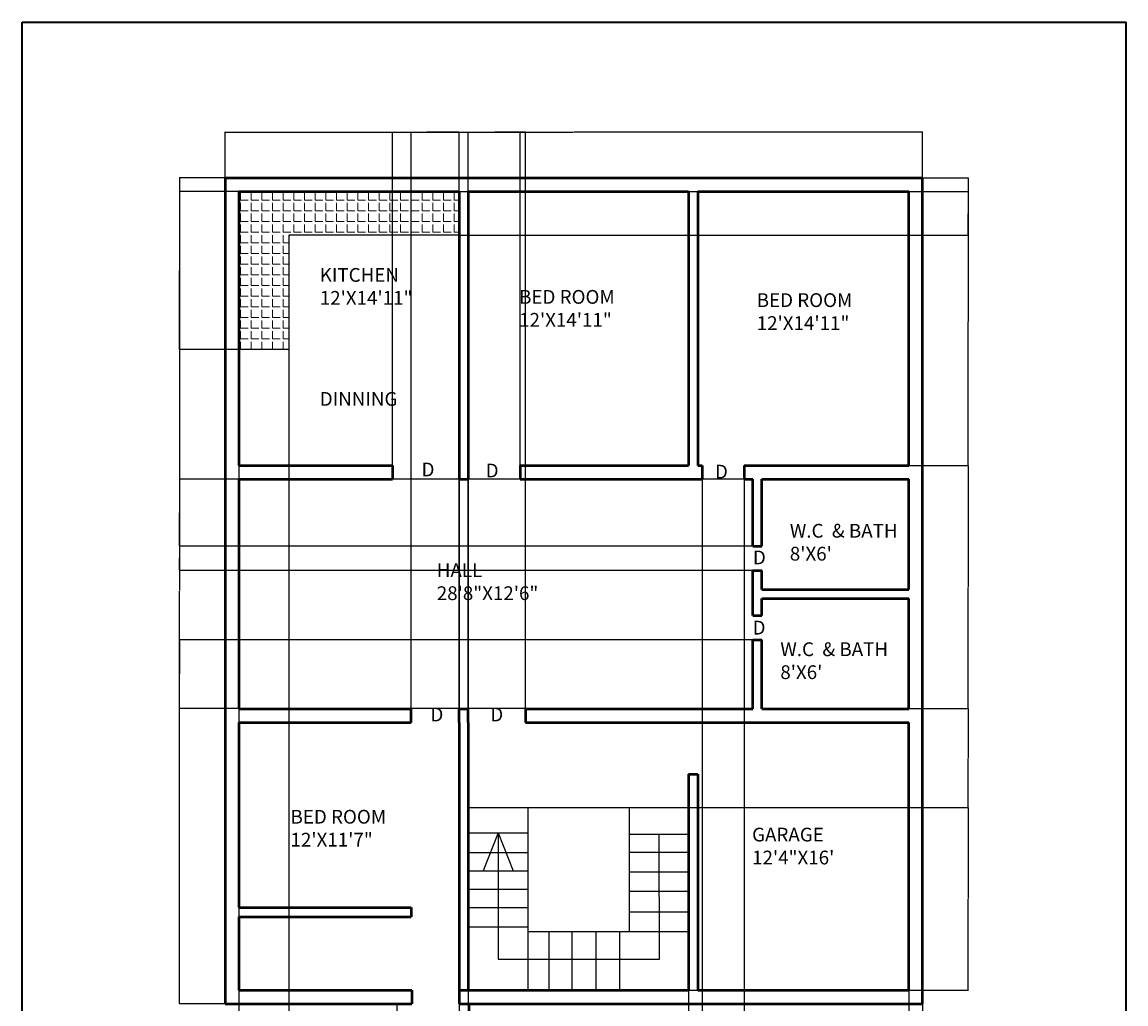
# Model space of a CAD drawing. Units: feet. Extents: x 3406 to 4127, y 2162 to 3204.
# Tile 3 of 3: x 3406 to 4127, y 2562 to 3204. Entities that reach past the tile are written whole.
import ezdxf

# ---------------------------------------------------------------- set-up
doc = ezdxf.new("R2010")
doc.units = ezdxf.units.FT
for name, color, linetype, lineweight in [('A-ANNO-DIMS', 2, 'Continuous', 18), ('A-ANNO-TEXT', 7, 'Continuous', 18), ('A-ANNO-TTLB', 7, 'Continuous', 35), ('A-AREA-IDEN', 7, 'Continuous', 18), ('A-FLOR-FIXT', 8, 'Continuous', 25), ('A-FLOR-FIXT-PATT', 9, 'Continuous', 13), ('A-FLOR-STRS', 7, 'Continuous', 25), ('A-WALL', 7, 'Continuous', 50)]:
    doc.layers.add(name, color=color, linetype=linetype, lineweight=lineweight)
doc.styles.get("Standard").update_dxf_attribs({"font": 'arial.ttf'})
doc.dimstyles.get("Standard").update_dxf_attribs({"dimtxt": 0.18, "dimasz": 0.18, "dimexe": 0.18, "dimexo": 0.0625, "dimgap": 0.09, "dimtad": 0, "dimtih": 1, "dimtoh": 1, "dimdec": 4, "dimzin": 0, "dimdsep": 46, "dimtxsty": 'Standard', "dimcen": 0.09, "dimadec": 0, "dimazin": 0, "dimtfac": 1, "dimtdec": 4, "dimtofl": 0, "dimtmove": 0, "dimatfit": 3, "dimfxl": 1, "dimtolj": 1, "dimtzin": 0, "dimarcsym": 0})

# ---------------------------------------------------------------- blocks, each defined once
blk = doc.blocks.new('*D4')
at = {"layer": 'A-ANNO-DIMS', "color": 0, "lineweight": -2, "transparency": 16777216}
for p, q in [((3538.39, 3101.97), (3538.39, 3131.89)), ((3994.39, 3101.97), (3994.39, 3131.89)), ((3538.57, 3131.71), (3766.1, 3131.71)), ((3994.21, 3131.71), (3766.68, 3131.71))]:
    blk.add_line(p, q, dxfattribs=at)
at = {"layer": 'A-ANNO-DIMS', "color": 0, "transparency": 16777216}
for points in [[(3538.57, 3131.74), (3538.57, 3131.68), (3538.39, 3131.71)], [(3994.21, 3131.74), (3994.21, 3131.68), (3994.39, 3131.71)]]:
    blk.add_solid(points, dxfattribs=at)
at = {"layer": 'Defpoints', "color": 0, "transparency": 16777216}
for p in [(3994.39, 3131.71), (3538.39, 3101.91), (3994.39, 3101.91)]:
    blk.add_point(p, dxfattribs=at)
at = {"layer": 'A-ANNO-DIMS', "color": 0, "transparency": 16777216, "insert": (3766.39, 3131.71), "char_height": 0.18, "attachment_point": 5}
blk.add_mtext('\\A1;456', dxfattribs=at)
blk = doc.blocks.new('*D5')
at = {"layer": 'A-ANNO-DIMS', "color": 0, "lineweight": -2, "transparency": 16777216}
for p, q in [((3538.33, 3101.91), (3508.41, 3101.91)), ((3508.59, 3101.73), (3508.59, 2832.09)), ((3508.59, 2562.09), (3508.59, 2831.72)), ((3538.33, 2561.91), (3508.41, 2561.91))]:
    blk.add_line(p, q, dxfattribs=at)
at = {"layer": 'A-ANNO-DIMS', "color": 0, "transparency": 16777216}
for points in [[(3508.56, 3101.73), (3508.62, 3101.73), (3508.59, 3101.91)], [(3508.56, 2562.09), (3508.62, 2562.09), (3508.59, 2561.91)]]:
    blk.add_solid(points, dxfattribs=at)
at = {"layer": 'Defpoints', "color": 0, "transparency": 16777216}
for p in [(3538.39, 3101.91), (3508.59, 2561.91), (3538.39, 2561.91)]:
    blk.add_point(p, dxfattribs=at)
at = {"layer": 'A-ANNO-DIMS', "color": 0, "transparency": 16777216, "insert": (3508.59, 2831.91), "char_height": 0.18, "attachment_point": 5}
blk.add_mtext('\\A1;540', dxfattribs=at)
blk = doc.blocks.new('*D9')
at = {"layer": 'A-ANNO-DIMS', "color": 0, "lineweight": -2, "transparency": 16777216}
for p, q in [((3841.39, 2570.84), (3841.39, 2509.54)), ((3985.39, 2570.84), (3985.39, 2509.54)), ((3841.57, 2509.72), (3913.11, 2509.72)), ((3985.21, 2509.72), (3913.67, 2509.72))]:
    blk.add_line(p, q, dxfattribs=at)
at = {"layer": 'A-ANNO-DIMS', "color": 0, "transparency": 16777216}
for points in [[(3841.57, 2509.75), (3841.57, 2509.69), (3841.39, 2509.72)], [(3985.21, 2509.75), (3985.21, 2509.69), (3985.39, 2509.72)]]:
    blk.add_solid(points, dxfattribs=at)
at = {"layer": 'Defpoints', "color": 0, "transparency": 16777216}
for p in [(3841.39, 2570.91), (3985.39, 2570.91), (3985.39, 2509.72)]:
    blk.add_point(p, dxfattribs=at)
at = {"layer": 'A-ANNO-DIMS', "color": 0, "transparency": 16777216, "insert": (3913.39, 2509.72), "char_height": 0.18, "attachment_point": 5}
blk.add_mtext('\\A1;144', dxfattribs=at)
blk = doc.blocks.new('*D10')
at = {"layer": 'A-ANNO-DIMS', "color": 0, "lineweight": -2, "transparency": 16777216}
for p, q in [((3994.45, 3101.91), (4024.37, 3101.91)), ((4024.19, 3101.73), (4024.19, 3008.09)), ((4024.19, 2914.09), (4024.19, 3007.72)), ((3985.45, 2913.91), (4024.37, 2913.91))]:
    blk.add_line(p, q, dxfattribs=at)
at = {"layer": 'A-ANNO-DIMS', "color": 0, "transparency": 16777216}
for points in [[(4024.16, 3101.73), (4024.22, 3101.73), (4024.19, 3101.91)], [(4024.16, 2914.09), (4024.22, 2914.09), (4024.19, 2913.91)]]:
    blk.add_solid(points, dxfattribs=at)
at = {"layer": 'Defpoints', "color": 0, "transparency": 16777216}
for p in [(3994.39, 3101.91), (3985.39, 2913.91), (4024.19, 2913.91)]:
    blk.add_point(p, dxfattribs=at)
at = {"layer": 'A-ANNO-DIMS', "color": 0, "transparency": 16777216, "insert": (4024.19, 3007.91), "char_height": 0.18, "attachment_point": 5}
blk.add_mtext('\\A1;188', dxfattribs=at)
blk = doc.blocks.new('*D11')
at = {"layer": 'A-ANNO-DIMS', "color": 0, "lineweight": -2, "transparency": 16777216}
for p, q in [((3985.45, 2913.91), (4024.37, 2913.91)), ((4024.19, 2913.73), (4024.19, 2834.59)), ((4024.19, 2755.09), (4024.19, 2834.22)), ((3985.45, 2754.91), (4024.37, 2754.91))]:
    blk.add_line(p, q, dxfattribs=at)
at = {"layer": 'A-ANNO-DIMS', "color": 0, "transparency": 16777216}
for points in [[(4024.16, 2913.73), (4024.22, 2913.73), (4024.19, 2913.91)], [(4024.16, 2755.09), (4024.22, 2755.09), (4024.19, 2754.91)]]:
    blk.add_solid(points, dxfattribs=at)
at = {"layer": 'Defpoints', "color": 0, "transparency": 16777216}
for p in [(3985.39, 2913.91), (3985.39, 2754.91), (4024.19, 2754.91)]:
    blk.add_point(p, dxfattribs=at)
at = {"layer": 'A-ANNO-DIMS', "color": 0, "transparency": 16777216, "insert": (4024.19, 2834.41), "char_height": 0.18, "attachment_point": 5}
blk.add_mtext('\\A1;159', dxfattribs=at)
blk = doc.blocks.new('*D12')
at = {"layer": 'A-ANNO-DIMS', "color": 0, "lineweight": -2, "transparency": 16777216}
for p, q in [((3841.45, 2690.33), (4024.37, 2690.33)), ((4024.19, 2690.15), (4024.19, 2630.8)), ((4024.19, 2571.09), (4024.19, 2630.43)), ((3841.45, 2570.91), (4024.37, 2570.91))]:
    blk.add_line(p, q, dxfattribs=at)
at = {"layer": 'A-ANNO-DIMS', "color": 0, "transparency": 16777216}
for points in [[(4024.16, 2690.15), (4024.22, 2690.15), (4024.19, 2690.33)], [(4024.16, 2571.09), (4024.22, 2571.09), (4024.19, 2570.91)]]:
    blk.add_solid(points, dxfattribs=at)
at = {"layer": 'Defpoints', "color": 0, "transparency": 16777216}
for p in [(3841.39, 2690.33), (4024.19, 2690.33), (3841.39, 2570.91)]:
    blk.add_point(p, dxfattribs=at)
at = {"layer": 'A-ANNO-DIMS', "color": 0, "transparency": 16777216, "insert": (4024.19, 2630.62), "char_height": 0.18, "attachment_point": 5}
blk.add_mtext('\\A1;119.42', dxfattribs=at)
blk = doc.blocks.new('*D13')
at = {"layer": 'A-ANNO-DIMS', "color": 0, "lineweight": -2, "transparency": 16777216}
for p, q in [((3985.45, 2754.91), (4024.37, 2754.91)), ((4024.19, 2754.73), (4024.19, 2722.8)), ((4024.19, 2690.51), (4024.19, 2722.43)), ((3841.45, 2690.33), (4024.37, 2690.33))]:
    blk.add_line(p, q, dxfattribs=at)
at = {"layer": 'A-ANNO-DIMS', "color": 0, "transparency": 16777216}
for points in [[(4024.16, 2754.73), (4024.22, 2754.73), (4024.19, 2754.91)], [(4024.16, 2690.51), (4024.22, 2690.51), (4024.19, 2690.33)]]:
    blk.add_solid(points, dxfattribs=at)
at = {"layer": 'Defpoints', "color": 0, "transparency": 16777216}
for p in [(3985.39, 2754.91), (4024.19, 2754.91), (3841.39, 2690.33)]:
    blk.add_point(p, dxfattribs=at)
at = {"layer": 'A-ANNO-DIMS', "color": 0, "transparency": 16777216, "insert": (4024.19, 2722.62), "char_height": 0.18, "attachment_point": 5}
blk.add_mtext('\\A1;64.58', dxfattribs=at)
blk = doc.blocks.new('*D14')
at = {"layer": 'A-ANNO-DIMS', "color": 0, "lineweight": -2, "transparency": 16777216}
for p, q in [((3647.87, 2913.97), (3647.87, 3131.89)), ((3691.39, 2913.97), (3691.39, 3131.89)), ((3648.05, 3131.71), (3669.23, 3131.71)), ((3691.21, 3131.71), (3670.03, 3131.71))]:
    blk.add_line(p, q, dxfattribs=at)
at = {"layer": 'A-ANNO-DIMS', "color": 0, "transparency": 16777216}
for points in [[(3648.05, 3131.74), (3648.05, 3131.68), (3647.87, 3131.71)], [(3691.21, 3131.74), (3691.21, 3131.68), (3691.39, 3131.71)]]:
    blk.add_solid(points, dxfattribs=at)
at = {"layer": 'Defpoints', "color": 0, "transparency": 16777216}
for p in [(3691.39, 3131.71), (3647.87, 2913.91), (3691.39, 2913.91)]:
    blk.add_point(p, dxfattribs=at)
at = {"layer": 'A-ANNO-DIMS', "color": 0, "transparency": 16777216, "insert": (3669.63, 3131.71), "char_height": 0.18, "attachment_point": 5}
blk.add_mtext('\\A1;43.52', dxfattribs=at)
blk = doc.blocks.new('*D15')
at = {"layer": 'A-ANNO-DIMS', "color": 0, "lineweight": -2, "transparency": 16777216}
for p, q in [((3697.39, 2913.97), (3697.39, 3131.89)), ((3731.22, 2913.97), (3731.22, 3131.89)), ((3697.57, 3131.71), (3713.91, 3131.71)), ((3731.04, 3131.71), (3714.7, 3131.71))]:
    blk.add_line(p, q, dxfattribs=at)
at = {"layer": 'A-ANNO-DIMS', "color": 0, "transparency": 16777216}
for points in [[(3697.57, 3131.74), (3697.57, 3131.68), (3697.39, 3131.71)], [(3731.04, 3131.74), (3731.04, 3131.68), (3731.22, 3131.71)]]:
    blk.add_solid(points, dxfattribs=at)
at = {"layer": 'Defpoints', "color": 0, "transparency": 16777216}
for p in [(3731.22, 3131.71), (3697.39, 2913.91), (3731.22, 2913.91)]:
    blk.add_point(p, dxfattribs=at)
at = {"layer": 'A-ANNO-DIMS', "color": 0, "transparency": 16777216, "insert": (3714.3, 3131.71), "char_height": 0.18, "attachment_point": 5}
blk.add_mtext('\\A1;33.83', dxfattribs=at)
blk = doc.blocks.new('*D16')
at = {"layer": 'A-ANNO-DIMS', "color": 0, "lineweight": -2, "transparency": 16777216}
for p, q in [((3850.19, 2904.84), (3850.19, 2509.54)), ((3877.72, 2904.84), (3877.72, 2509.54)), ((3850.37, 2509.72), (3863.49, 2509.72)), ((3877.54, 2509.72), (3864.42, 2509.72))]:
    blk.add_line(p, q, dxfattribs=at)
at = {"layer": 'A-ANNO-DIMS', "color": 0, "transparency": 16777216}
for points in [[(3850.37, 2509.75), (3850.37, 2509.69), (3850.19, 2509.72)], [(3877.54, 2509.75), (3877.54, 2509.69), (3877.72, 2509.72)]]:
    blk.add_solid(points, dxfattribs=at)
at = {"layer": 'Defpoints', "color": 0, "transparency": 16777216}
for p in [(3850.19, 2904.91), (3877.72, 2904.91), (3877.72, 2509.72)]:
    blk.add_point(p, dxfattribs=at)
at = {"layer": 'A-ANNO-DIMS', "color": 0, "transparency": 16777216, "insert": (3863.95, 2509.72), "char_height": 0.18, "attachment_point": 5}
blk.add_mtext('\\A1;27.533', dxfattribs=at)
blk = doc.blocks.new('*D17')
at = {"layer": 'A-ANNO-DIMS', "color": 0, "lineweight": -2, "transparency": 16777216}
for p, q in [((3660.15, 2754.97), (3660.15, 3131.89)), ((3691.39, 2754.97), (3691.39, 3131.89)), ((3660.33, 3131.71), (3675.38, 3131.71)), ((3691.21, 3131.71), (3676.17, 3131.71))]:
    blk.add_line(p, q, dxfattribs=at)
at = {"layer": 'A-ANNO-DIMS', "color": 0, "transparency": 16777216}
for points in [[(3660.33, 3131.74), (3660.33, 3131.68), (3660.15, 3131.71)], [(3691.21, 3131.74), (3691.21, 3131.68), (3691.39, 3131.71)]]:
    blk.add_solid(points, dxfattribs=at)
at = {"layer": 'Defpoints', "color": 0, "transparency": 16777216}
for p in [(3691.39, 3131.71), (3660.15, 2754.91), (3691.39, 2754.91)]:
    blk.add_point(p, dxfattribs=at)
at = {"layer": 'A-ANNO-DIMS', "color": 0, "transparency": 16777216, "insert": (3675.77, 3131.71), "char_height": 0.18, "attachment_point": 5}
blk.add_mtext('\\A1;31.24', dxfattribs=at)
blk = doc.blocks.new('*D18')
at = {"layer": 'A-ANNO-DIMS', "color": 0, "lineweight": -2, "transparency": 16777216}
for p, q in [((3697.39, 2754.97), (3697.39, 3131.89)), ((3734.88, 2754.97), (3734.88, 3131.89)), ((3697.57, 3131.71), (3715.67, 3131.71)), ((3734.7, 3131.71), (3716.6, 3131.71))]:
    blk.add_line(p, q, dxfattribs=at)
at = {"layer": 'A-ANNO-DIMS', "color": 0, "transparency": 16777216}
for points in [[(3697.57, 3131.74), (3697.57, 3131.68), (3697.39, 3131.71)], [(3734.7, 3131.74), (3734.7, 3131.68), (3734.88, 3131.71)]]:
    blk.add_solid(points, dxfattribs=at)
at = {"layer": 'Defpoints', "color": 0, "transparency": 16777216}
for p in [(3734.88, 3131.71), (3697.39, 2754.91), (3734.88, 2754.91)]:
    blk.add_point(p, dxfattribs=at)
at = {"layer": 'A-ANNO-DIMS', "color": 0, "transparency": 16777216, "insert": (3716.13, 3131.71), "char_height": 0.18, "attachment_point": 5}
blk.add_mtext('\\A1;37.485', dxfattribs=at)
blk = doc.blocks.new('*D19')
at = {"layer": 'A-ANNO-DIMS', "color": 0, "lineweight": -2, "transparency": 16777216}
for p, q in [((3883.33, 2861.21), (3508.41, 2861.21)), ((3508.59, 2861.03), (3508.59, 2853.4)), ((3508.59, 2845.41), (3508.59, 2853.03)), ((3883.33, 2845.23), (3508.41, 2845.23))]:
    blk.add_line(p, q, dxfattribs=at)
at = {"layer": 'A-ANNO-DIMS', "color": 0, "transparency": 16777216}
for points in [[(3508.56, 2861.03), (3508.62, 2861.03), (3508.59, 2861.21)], [(3508.56, 2845.41), (3508.62, 2845.41), (3508.59, 2845.23)]]:
    blk.add_solid(points, dxfattribs=at)
at = {"layer": 'Defpoints', "color": 0, "transparency": 16777216}
for p in [(3508.59, 2861.21), (3883.39, 2861.21), (3883.39, 2845.23)]:
    blk.add_point(p, dxfattribs=at)
at = {"layer": 'A-ANNO-DIMS', "color": 0, "transparency": 16777216, "insert": (3508.59, 2853.22), "char_height": 0.18, "attachment_point": 5}
blk.add_mtext('\\A1;15.98', dxfattribs=at)
blk = doc.blocks.new('*D20')
at = {"layer": 'A-ANNO-DIMS', "color": 0, "lineweight": -2, "transparency": 16777216}
for p, q in [((3883.33, 2904.91), (3508.41, 2904.91)), ((3508.59, 2904.73), (3508.59, 2883.24)), ((3508.59, 2861.39), (3508.59, 2882.87)), ((3883.33, 2861.21), (3508.41, 2861.21))]:
    blk.add_line(p, q, dxfattribs=at)
at = {"layer": 'A-ANNO-DIMS', "color": 0, "transparency": 16777216}
for points in [[(3508.56, 2904.73), (3508.62, 2904.73), (3508.59, 2904.91)], [(3508.56, 2861.39), (3508.62, 2861.39), (3508.59, 2861.21)]]:
    blk.add_solid(points, dxfattribs=at)
at = {"layer": 'Defpoints', "color": 0, "transparency": 16777216}
for p in [(3883.39, 2904.91), (3508.59, 2861.21), (3883.39, 2861.21)]:
    blk.add_point(p, dxfattribs=at)
at = {"layer": 'A-ANNO-DIMS', "color": 0, "transparency": 16777216, "insert": (3508.59, 2883.06), "char_height": 0.18, "attachment_point": 5}
blk.add_mtext('\\A1;43.7', dxfattribs=at)
blk = doc.blocks.new('*D21')
at = {"layer": 'A-ANNO-DIMS', "color": 0, "lineweight": -2, "transparency": 16777216}
for p, q in [((3883.33, 2799.89), (3508.41, 2799.89)), ((3508.59, 2799.71), (3508.59, 2777.58)), ((3508.59, 2755.09), (3508.59, 2777.22)), ((3883.33, 2754.91), (3508.41, 2754.91))]:
    blk.add_line(p, q, dxfattribs=at)
at = {"layer": 'A-ANNO-DIMS', "color": 0, "transparency": 16777216}
for points in [[(3508.56, 2799.71), (3508.62, 2799.71), (3508.59, 2799.89)], [(3508.56, 2755.09), (3508.62, 2755.09), (3508.59, 2754.91)]]:
    blk.add_solid(points, dxfattribs=at)
at = {"layer": 'Defpoints', "color": 0, "transparency": 16777216}
for p in [(3508.59, 2799.89), (3883.39, 2799.89), (3883.39, 2754.91)]:
    blk.add_point(p, dxfattribs=at)
at = {"layer": 'A-ANNO-DIMS', "color": 0, "transparency": 16777216, "insert": (3508.59, 2777.4), "char_height": 0.18, "attachment_point": 5}
blk.add_mtext('\\A1;44.98', dxfattribs=at)
blk = doc.blocks.new('*D22')
at = {"layer": 'A-ANNO-DIMS', "color": 0, "lineweight": -2, "transparency": 16777216}
for p, q in [((3985.39, 2570.84), (3985.39, 2509.54)), ((3994.39, 2561.84), (3994.39, 2509.54)), ((3985.57, 2509.72), (3989.74, 2509.72)), ((3994.21, 2509.72), (3990.04, 2509.72))]:
    blk.add_line(p, q, dxfattribs=at)
at = {"layer": 'A-ANNO-DIMS', "color": 0, "transparency": 16777216}
for points in [[(3985.57, 2509.75), (3985.57, 2509.69), (3985.39, 2509.72)], [(3994.21, 2509.75), (3994.21, 2509.69), (3994.39, 2509.72)]]:
    blk.add_solid(points, dxfattribs=at)
at = {"layer": 'Defpoints', "color": 0, "transparency": 16777216}
for p in [(3985.39, 2570.91), (3994.39, 2561.91), (3985.39, 2509.72)]:
    blk.add_point(p, dxfattribs=at)
at = {"layer": 'A-ANNO-DIMS', "color": 0, "transparency": 16777216, "insert": (3989.89, 2509.72), "char_height": 0.18, "attachment_point": 5}
blk.add_mtext('\\A1;9', dxfattribs=at)
blk = doc.blocks.new('*D23')
at = {"layer": 'A-ANNO-DIMS', "color": 0, "lineweight": -2, "transparency": 16777216}
for p, q in [((3691.39, 3092.84), (3691.39, 2509.54)), ((3697.39, 3092.84), (3697.39, 2509.54)), ((3691.57, 2509.72), (3694.24, 2509.72)), ((3697.21, 2509.72), (3694.54, 2509.72))]:
    blk.add_line(p, q, dxfattribs=at)
at = {"layer": 'A-ANNO-DIMS', "color": 0, "transparency": 16777216}
for points in [[(3691.57, 2509.75), (3691.57, 2509.69), (3691.39, 2509.72)], [(3697.21, 2509.75), (3697.21, 2509.69), (3697.39, 2509.72)]]:
    blk.add_solid(points, dxfattribs=at)
at = {"layer": 'Defpoints', "color": 0, "transparency": 16777216}
for p in [(3691.39, 3092.91), (3697.39, 3092.91), (3697.39, 2509.72)]:
    blk.add_point(p, dxfattribs=at)
at = {"layer": 'A-ANNO-DIMS', "color": 0, "transparency": 16777216, "insert": (3694.39, 2509.72), "char_height": 0.18, "attachment_point": 5}
blk.add_mtext('\\A1;6', dxfattribs=at)
blk = doc.blocks.new('*D24')
at = {"layer": 'A-ANNO-DIMS', "color": 0, "lineweight": -2, "transparency": 16777216}
for p, q in [((3547.39, 2989.54), (3547.39, 2509.54)), ((3580.04, 2989.54), (3580.04, 2509.54)), ((3547.57, 2509.72), (3563.25, 2509.72)), ((3579.86, 2509.72), (3564.18, 2509.72))]:
    blk.add_line(p, q, dxfattribs=at)
at = {"layer": 'A-ANNO-DIMS', "color": 0, "transparency": 16777216}
for points in [[(3547.57, 2509.75), (3547.57, 2509.69), (3547.39, 2509.72)], [(3579.86, 2509.75), (3579.86, 2509.69), (3580.04, 2509.72)]]:
    blk.add_solid(points, dxfattribs=at)
at = {"layer": 'Defpoints', "color": 0, "transparency": 16777216}
for p in [(3547.39, 2989.6), (3580.04, 2989.6), (3580.04, 2509.72)]:
    blk.add_point(p, dxfattribs=at)
at = {"layer": 'A-ANNO-DIMS', "color": 0, "transparency": 16777216, "insert": (3563.71, 2509.72), "char_height": 0.18, "attachment_point": 5}
blk.add_mtext('\\A1;32.646', dxfattribs=at)
blk = doc.blocks.new('*D25')
at = {"layer": 'A-ANNO-DIMS', "color": 0, "lineweight": -2, "transparency": 16777216}
for p, q in [((3547.33, 3092.91), (3508.41, 3092.91)), ((3508.59, 3092.73), (3508.59, 3041.44)), ((3508.59, 2989.78), (3508.59, 3041.07)), ((3547.33, 2989.6), (3508.41, 2989.6))]:
    blk.add_line(p, q, dxfattribs=at)
at = {"layer": 'A-ANNO-DIMS', "color": 0, "transparency": 16777216}
for points in [[(3508.56, 3092.73), (3508.62, 3092.73), (3508.59, 3092.91)], [(3508.56, 2989.78), (3508.62, 2989.78), (3508.59, 2989.6)]]:
    blk.add_solid(points, dxfattribs=at)
at = {"layer": 'Defpoints', "color": 0, "transparency": 16777216}
for p in [(3508.59, 3092.91), (3547.39, 3092.91), (3547.39, 2989.6)]:
    blk.add_point(p, dxfattribs=at)
at = {"layer": 'A-ANNO-DIMS', "color": 0, "transparency": 16777216, "insert": (3508.59, 3041.25), "char_height": 0.18, "attachment_point": 5}
blk.add_mtext('\\A1;103.3', dxfattribs=at)
blk = doc.blocks.new('*D26')
at = {"layer": 'A-ANNO-DIMS', "color": 0, "lineweight": -2, "transparency": 16777216}
for p, q in [((3691.45, 3092.91), (4024.37, 3092.91)), ((4024.19, 3092.73), (4024.19, 3078.84)), ((4024.19, 3064.59), (4024.19, 3078.48)), ((3691.45, 3064.41), (4024.37, 3064.41))]:
    blk.add_line(p, q, dxfattribs=at)
at = {"layer": 'A-ANNO-DIMS', "color": 0, "transparency": 16777216}
for points in [[(4024.16, 3092.73), (4024.22, 3092.73), (4024.19, 3092.91)], [(4024.16, 3064.59), (4024.22, 3064.59), (4024.19, 3064.41)]]:
    blk.add_solid(points, dxfattribs=at)
at = {"layer": 'Defpoints', "color": 0, "transparency": 16777216}
for p in [(3691.39, 3092.91), (3691.39, 3064.41), (4024.19, 3064.41)]:
    blk.add_point(p, dxfattribs=at)
at = {"layer": 'A-ANNO-DIMS', "color": 0, "transparency": 16777216, "insert": (4024.19, 3078.66), "char_height": 0.18, "attachment_point": 5}
blk.add_mtext('\\A1;28.494', dxfattribs=at)

msp = doc.modelspace()

# ---------------------------------------------------------------- hatches: boundary and pattern name
at = {"layer": 'A-FLOR-FIXT-PATT'}
h = msp.add_hatch(dxfattribs=at)
h.set_pattern_fill('ANGLE', color=256)
h.set_pattern_definition([(0, (0, 0), (0, 6.985), [5.08, -1.905]), (90, (0, 0), (-6.985, 4e-16), [5.08, -1.905])])
h.paths.add_polyline_path([(3691.3916, 3092.9057), (3547.3916, 3092.9057), (3547.3916, 2989.6004), (3580.0374, 2989.6004), (3580.0374, 3064.4115), (3691.3916, 3064.4115)])

# ---------------------------------------------------------------- linework, layer by layer
at = {"layer": 'A-ANNO-TTLB'}
msp.add_lwpolyline([(3405.6917, 3203.7208), (4127.2965, 3203.7208), (4127.2965, 2161.7472), (3405.6917, 2161.7472)], close=True, dxfattribs=at)
at = {"layer": 'A-FLOR-FIXT'}
for p, q in [((3691.3916, 3064.4115), (3580.0374, 3064.4115)), ((3580.0374, 3064.4115), (3580.0374, 2989.6004)), ((3580.0374, 2989.6004), (3547.3916, 2989.6004))]:
    msp.add_line(p, q, dxfattribs=at)
at = {"layer": 'A-FLOR-STRS'}
for p, q in [((3697.3916, 2690.3252), (3841.3916, 2690.3252)), ((3736.2793, 2690.3252), (3736.2793, 2609.1556)), ((3802.8179, 2609.1556), (3802.8179, 2690.3252)), ((3697.3916, 2673.6483), (3736.2793, 2673.6483)), ((3716.8355, 2673.6483), (3707.0405, 2648.9918)), ((3716.8355, 2673.6483), (3716.8355, 2591.2563)), ((3716.8355, 2673.6483), (3726.7901, 2648.9918)), ((3802.8179, 2672.8187), (3841.3916, 2672.8187)), ((3822.3962, 2591.2563), (3822.1047, 2672.8187)), ((3697.3916, 2660.9678), (3736.2793, 2660.9678)), ((3802.8179, 2661.1621), (3841.3916, 2661.1621)), ((3697.3916, 2648.9918), (3736.2793, 2648.9918)), ((3802.8179, 2648.1605), (3841.3916, 2648.1605)), ((3697.3916, 2637.0158), (3736.2793, 2637.0158)), ((3802.8179, 2635.6072), (3841.3916, 2635.6072)), ((3697.3916, 2625.0398), (3736.2793, 2625.0398)), ((3802.8179, 2622.1572), (3841.3916, 2622.1572)), ((3697.3916, 2612.3593), (3736.2793, 2612.3593)), ((3736.2793, 2609.1556), (3802.8179, 2609.1556)), ((3736.2793, 2609.1556), (3736.2793, 2570.9057)), ((3750.0515, 2609.1556), (3750.0515, 2570.9057)), ((3765.1564, 2609.1556), (3765.1564, 2570.9057)), ((3780.7056, 2609.1556), (3780.7056, 2570.9057)), ((3796.2548, 2609.1556), (3796.2548, 2570.9057)), ((3802.8179, 2609.1556), (3841.3916, 2609.1556)), ((3716.8355, 2591.2563), (3822.3962, 2591.2563)), ((3650.6189, 2561.9057), (3650.6189, 2539.5223)), ((3698.33, 2539.5223), (3698.33, 2561.9057))]:
    msp.add_line(p, q, dxfattribs=at)
at = {"layer": 'A-WALL'}
for p, q in [((3538.3916, 3101.9057), (3994.3916, 3101.9057)), ((3538.3916, 3101.9057), (3538.3916, 2561.9057)), ((3994.3916, 2561.9057), (3994.3916, 3101.9057)), ((3547.3916, 3092.9057), (3547.3916, 2913.9057)), ((3547.3916, 3092.9057), (3691.3916, 3092.9057)), ((3691.3916, 3092.9057), (3691.3916, 2913.9057)), ((3697.3916, 3092.9057), (3697.3916, 2913.9057)), ((3697.3916, 3092.9057), (3841.3916, 3092.9057)), ((3841.3916, 3092.9057), (3841.3916, 2913.9057)), ((3847.3916, 3092.9057), (3847.3916, 2913.9057)), ((3847.3916, 3092.9057), (3985.3916, 3092.9057)), ((3985.3916, 2913.9057), (3985.3916, 3092.9057)), ((3547.3916, 2913.9057), (3647.8694, 2913.9057)), ((3647.8694, 2913.9057), (3647.8694, 2904.9057)), ((3691.3916, 2913.9057), (3691.3916, 2904.9057)), ((3697.3916, 2913.9057), (3697.3916, 2904.9057)), ((3731.2184, 2913.9057), (3731.2184, 2904.9057)), ((3731.2184, 2913.9057), (3841.3916, 2913.9057)), ((3847.3916, 2913.9057), (3850.1884, 2913.9057)), ((3850.1884, 2913.9057), (3850.1884, 2904.9057)), ((3877.7214, 2913.9057), (3877.7214, 2904.9057)), ((3877.7214, 2913.9057), (3985.3916, 2913.9057)), ((3547.3916, 2904.9057), (3647.8694, 2904.9057)), ((3547.3916, 2904.9057), (3547.3916, 2754.9057)), ((3691.3916, 2904.9057), (3697.3916, 2904.9057)), ((3731.2184, 2904.9057), (3850.1884, 2904.9057)), ((3877.7214, 2904.9057), (3883.3916, 2904.9057)), ((3883.3916, 2861.205), (3883.3916, 2904.9057)), ((3889.3916, 2861.205), (3889.3916, 2904.9057)), ((3889.3916, 2904.9057), (3985.3916, 2904.9057)), ((3985.3916, 2832.9057), (3985.3916, 2904.9057)), ((3883.3916, 2861.205), (3889.3916, 2861.205)), ((3883.3916, 2832.9057), (3883.3916, 2845.2257)), ((3883.3916, 2845.2257), (3889.3916, 2845.2257)), ((3889.3916, 2832.9057), (3889.3916, 2845.2257)), ((3883.3916, 2815.8683), (3883.3916, 2832.9057)), ((3889.3916, 2832.9057), (3985.3916, 2832.9057)), ((3889.3916, 2826.9057), (3985.3916, 2826.9057)), ((3889.3916, 2815.8683), (3889.3916, 2826.9057)), ((3985.3916, 2754.9057), (3985.3916, 2826.9057)), ((3883.3916, 2815.8683), (3889.3916, 2815.8683)), ((3883.3916, 2754.9057), (3883.3916, 2799.889)), ((3883.3916, 2799.889), (3889.3916, 2799.889)), ((3889.3916, 2754.9057), (3889.3916, 2799.889)), ((3547.3916, 2754.9057), (3660.153, 2754.9057)), ((3660.153, 2745.9057), (3660.153, 2754.9057)), ((3691.3916, 2745.9057), (3691.3916, 2754.9057)), ((3691.3916, 2754.9057), (3697.3916, 2754.9057)), ((3697.3916, 2745.9057), (3697.3916, 2754.9057)), ((3734.8765, 2754.9057), (3734.8765, 2745.9057)), ((3734.8765, 2754.9057), (3883.3916, 2754.9057)), ((3889.3916, 2754.9057), (3985.3916, 2754.9057)), ((3547.3916, 2745.9057), (3660.153, 2745.9057)), ((3547.3916, 2745.9057), (3547.3916, 2624.9057)), ((3691.3916, 2745.9057), (3691.3916, 2570.9057)), ((3697.3916, 2745.9057), (3697.3916, 2570.9057)), ((3734.8765, 2745.9057), (3985.3916, 2745.9057)), ((3985.3916, 2570.9057), (3985.3916, 2745.9057)), ((3841.3916, 2712.1157), (3841.3916, 2570.9057)), ((3841.3916, 2712.1157), (3847.3916, 2712.1157)), ((3847.3916, 2712.1157), (3847.3916, 2570.9057)), ((3547.3916, 2624.9057), (3660.153, 2624.9057)), ((3660.153, 2624.9057), (3660.153, 2618.9057)), ((3547.3916, 2618.9057), (3660.153, 2618.9057)), ((3547.3916, 2618.9057), (3547.3916, 2570.9057)), ((3547.3916, 2570.9057), (3660.5781, 2570.9057)), ((3660.5781, 2570.9057), (3660.5781, 2561.9057)), ((3691.3916, 2570.9057), (3691.3916, 2561.9057)), ((3691.3916, 2570.9057), (3697.3916, 2570.9057)), ((3697.3916, 2570.9057), (3841.3916, 2570.9057)), ((3847.3916, 2570.9057), (3985.3916, 2570.9057)), ((3538.3916, 2561.9057), (3660.5781, 2561.9057)), ((3691.3916, 2561.9057), (3994.3916, 2561.9057))]:
    msp.add_line(p, q, dxfattribs=at)

# ---------------------------------------------------------------- texts
at = {"layer": 'A-ANNO-TEXT', "char_height": 9, "attachment_point": 1}
for insert in [(3666.855, 2915.7455), (3708.7544, 2915.0535), (3858.6343, 2914.3512), (3883.4584, 2858.256), (3883.2516, 2812.3791), (3672.6304, 2755.5657), (3711.7975, 2755.5657)]:
    msp.add_mtext_dynamic_manual_height_columns('D', width=89.058037, gutter_width=12.5, heights=[0], dxfattribs=dict(at, insert=insert))
at = {"layer": 'A-AREA-IDEN', "char_height": 9, "attachment_point": 1}
for s, insert in [('KITCHEN\\P12\'X14\'11"', (3600.302, 3042.9368)), ('BED ROOM\\P12\'X14\'11"', (3730.6095, 3028.577)), ('BED ROOM\\P12\'X14\'11"', (3885.9474, 3026.4637)), ('DINNING', (3600.302, 2961.8896)), ("W.C  & BATH\\P8'X6'", (3907.5804, 2875.7087)), ('HALL\\P28\'8"X12\'6"', (3676.7912, 2849.8936)), ("W.C  & BATH\\P8'X6'", (3901.3651, 2798.2633)), ('BED ROOM\\P12\'X11\'7"', (3581.1715, 2688.7613)), ('GARAGE\\P12\'4"X16\'', (3882.9184, 2677.0897))]:
    msp.add_mtext_dynamic_manual_height_columns(s, width=89.058037, gutter_width=12.5, heights=[0], dxfattribs=dict(at, insert=insert))

# ---------------------------------------------------------------- dimensions: what is measured, and where the dimension line sits
at = {"layer": 'A-ANNO-DIMS'}
for base, p1, p2, override, picture, middle in [((3994.3916, 3131.7057), (3538.3916, 3101.9057), (3994.3916, 3101.9057), {"dimdec": 0, "dimlfac": 1, "dimrnd": 0, "dimzin": 0, "dimdsep": 46, "dimlunit": 2}, '*D4', (3766.3916, 3131.7057)), ((3691.3916, 3131.7057), (3647.8694, 2913.9057), (3691.3916, 2913.9057), {"dimdec": 2, "dimlfac": 1, "dimrnd": 0, "dimzin": 0, "dimdsep": 46, "dimlunit": 2}, '*D14', (3669.6305, 3131.7057)), ((3691.3916, 3131.7057), (3660.153, 2754.9057), (3691.3916, 2754.9057), {"dimdec": 2, "dimlfac": 1, "dimrnd": 0, "dimzin": 0, "dimdsep": 46, "dimlunit": 2}, '*D17', (3675.7723, 3131.7057)), ((3731.2184, 3131.7057), (3697.3916, 2913.9057), (3731.2184, 2913.9057), {"dimdec": 2, "dimlfac": 1, "dimrnd": 0, "dimzin": 0, "dimdsep": 46, "dimlunit": 2}, '*D15', (3714.305, 3131.7057)), ((3734.8765, 3131.7057), (3697.3916, 2754.9057), (3734.8765, 2754.9057), {"dimdec": 3, "dimlfac": 1, "dimrnd": 0, "dimzin": 0, "dimdsep": 46, "dimlunit": 2}, '*D18', (3716.1341, 3131.7057)), ((3697.3916, 2509.7223), (3691.3916, 3092.9057), (3697.3916, 3092.9057), {"dimdec": 0, "dimlfac": 1, "dimrnd": 0, "dimzin": 0, "dimdsep": 46, "dimlunit": 2}, '*D23', (3694.3916, 2509.7223)), ((3580.0374, 2509.7223), (3547.3916, 2989.6004), (3580.0374, 2989.6004), {"dimdec": 3, "dimlfac": 1, "dimrnd": 0, "dimzin": 0, "dimdsep": 46, "dimlunit": 2}, '*D24', (3563.7145, 2509.7223)), ((3877.7214, 2509.7223), (3850.1884, 2904.9057), (3877.7214, 2904.9057), {"dimdec": 3, "dimlfac": 1, "dimrnd": 0, "dimzin": 0, "dimdsep": 46, "dimlunit": 2}, '*D16', (3863.9549, 2509.7223)), ((3985.3916, 2509.7223), (3841.3916, 2570.9057), (3985.3916, 2570.9057), {"dimdec": 0, "dimlfac": 1, "dimrnd": 0, "dimzin": 0, "dimdsep": 46, "dimlunit": 2}, '*D9', (3913.3916, 2509.7223)), ((3985.3916, 2509.7223), (3994.3916, 2561.9057), (3985.3916, 2570.9057), {"dimdec": 0, "dimlfac": 1, "dimrnd": 0, "dimzin": 0, "dimdsep": 46, "dimlunit": 2}, '*D22', (3989.8916, 2509.7223))]:
    dim = msp.add_linear_dim(base=base, p1=p1, p2=p2, dimstyle='Standard', override=override, dxfattribs=at)
    dim.commit()
    dim.dimension.update_dxf_attribs({"geometry": picture, "text_midpoint": middle})
for base, p1, p2, override, picture, middle in [((3508.5916, 2561.9057), (3538.3916, 3101.9057), (3538.3916, 2561.9057), {"dimdec": 0, "dimlfac": 1, "dimrnd": 0, "dimzin": 0, "dimdsep": 46, "dimlunit": 2}, '*D5', (3508.5916, 2831.9057)), ((4024.1916, 2913.9057), (3994.3916, 3101.9057), (3985.3916, 2913.9057), {"dimdec": 0, "dimlfac": 1, "dimrnd": 0, "dimzin": 0, "dimdsep": 46, "dimlunit": 2}, '*D10', (4024.1916, 3007.9057)), ((3508.5916, 3092.9057), (3547.3916, 2989.6004), (3547.3916, 3092.9057), {"dimdec": 1, "dimlfac": 1, "dimrnd": 0, "dimzin": 0, "dimdsep": 46, "dimlunit": 2}, '*D25', (3508.5916, 3041.2531)), ((4024.1916, 3064.4115), (3691.3916, 3092.9057), (3691.3916, 3064.4115), {"dimdec": 3, "dimlfac": 1, "dimrnd": 0, "dimzin": 0, "dimdsep": 46, "dimlunit": 2}, '*D26', (4024.1916, 3078.6586)), ((4024.1916, 2754.9057), (3985.3916, 2913.9057), (3985.3916, 2754.9057), {"dimdec": 0, "dimlfac": 1, "dimrnd": 0, "dimzin": 0, "dimdsep": 46, "dimlunit": 2}, '*D11', (4024.1916, 2834.4057)), ((3508.5916, 2861.205), (3883.3916, 2904.9057), (3883.3916, 2861.205), {"dimdec": 1, "dimlfac": 1, "dimrnd": 0, "dimzin": 0, "dimdsep": 46, "dimlunit": 2}, '*D20', (3508.5916, 2883.0554)), ((3508.5916, 2861.205), (3883.3916, 2845.2257), (3883.3916, 2861.205), {"dimdec": 2, "dimlfac": 1, "dimrnd": 0, "dimzin": 0, "dimdsep": 46, "dimlunit": 2}, '*D19', (3508.5916, 2853.2154)), ((3508.5916, 2799.889), (3883.3916, 2754.9057), (3883.3916, 2799.889), {"dimdec": 2, "dimlfac": 1, "dimrnd": 0, "dimzin": 0, "dimdsep": 46, "dimlunit": 2}, '*D21', (3508.5916, 2777.3974)), ((4024.1916, 2754.9057), (3841.3916, 2690.3252), (3985.3916, 2754.9057), {"dimdec": 2, "dimlfac": 1, "dimrnd": 0, "dimzin": 0, "dimdsep": 46, "dimlunit": 2}, '*D13', (4024.1916, 2722.6155)), ((4024.1916, 2690.3252), (3841.3916, 2570.9057), (3841.3916, 2690.3252), {"dimdec": 2, "dimlfac": 1, "dimrnd": 0, "dimzin": 0, "dimdsep": 46, "dimlunit": 2}, '*D12', (4024.1916, 2630.6155))]:
    dim = msp.add_linear_dim(base=base, p1=p1, p2=p2, angle=90, dimstyle='Standard', override=override, dxfattribs=at)
    dim.commit()
    dim.dimension.update_dxf_attribs({"geometry": picture, "text_midpoint": middle})

doc.saveas('drawing.dxf')
